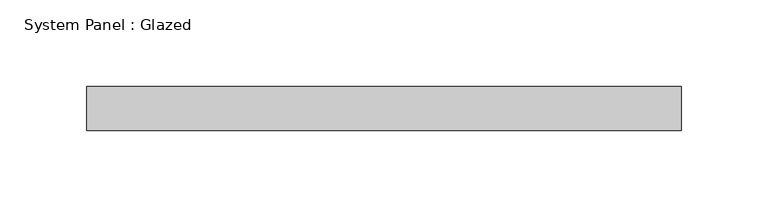
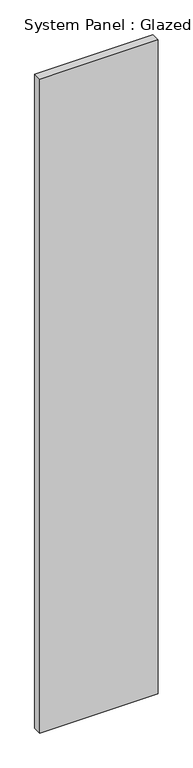
"""IFC4 building model written with IfcOpenShell, lengths in millimetres: plate geometry, System Panel : Glazed."""

from ifc_helpers import new_model, si_unit, origin, origin_with_axes, place, context, project, spatial, polyline, outline, extrude, source, transform, mapped, element, save


def system_panel_glazed_d43c1d57(model_context):
    return source(origin(), model_context, "Body", "SweptSolid", [
        extrude(outline(polyline([(171.45, 19.05), (-171.45, 19.05), (-171.45, 44.45), (171.45, 44.45), (171.45, 19.05)])), origin_with_axes(), (0.0, 0.0, 1.0), 2006.6),
    ])


if __name__ == "__main__":
    model = new_model("IFC4")
    model_context = context("Model", 3, world=origin())
    ifc_project = project(units=[si_unit("LENGTHUNIT", "METRE", prefix="MILLI")], contexts=[model_context])
    site = spatial("IfcSite", under=ifc_project)
    building = spatial("IfcBuilding", under=site)
    placement = place(None, origin())
    system_panel_glazed_shape = system_panel_glazed_d43c1d57(model_context)
    element("IfcPlate", 1, ObjectType="System Panel : Glazed", at=placement, inside=building, context=model_context, shape_type="MappedRepresentation", body=[
        mapped(system_panel_glazed_shape, transform((0.0, 0.0, 0.0), x_axis=(1.0, 0.0, 0.0), y_axis=(0.0, 1.0, 0.0), z_axis=(0.0, 0.0, 1.0))),
    ])
    save(model, "model.ifc")

# Revit data of these elements
# Type "System Panel : Glazed"
#   Construction Type Id = "GSP4R"
#   Analytic Construction = "1/8 in Pilkington single glazing"
#   Visual Light Transmittance = 0.9
#   Solar Heat Gain Coefficient = 0.86
#   Heat Transfer Coefficient (U) = 1.18115 BTU/(h·ft²·°F)
#   Define Thermal Properties by = 1
# Element 1 (IfcPlate, "System Panel : Glazed")
#   Materials on its faces: "Glass"
# Materials
#   "Glass": class "Glass", colour RGB 0 128 192, transparency 0.75, Description = "Soda Lime Glass", Cost = 0
